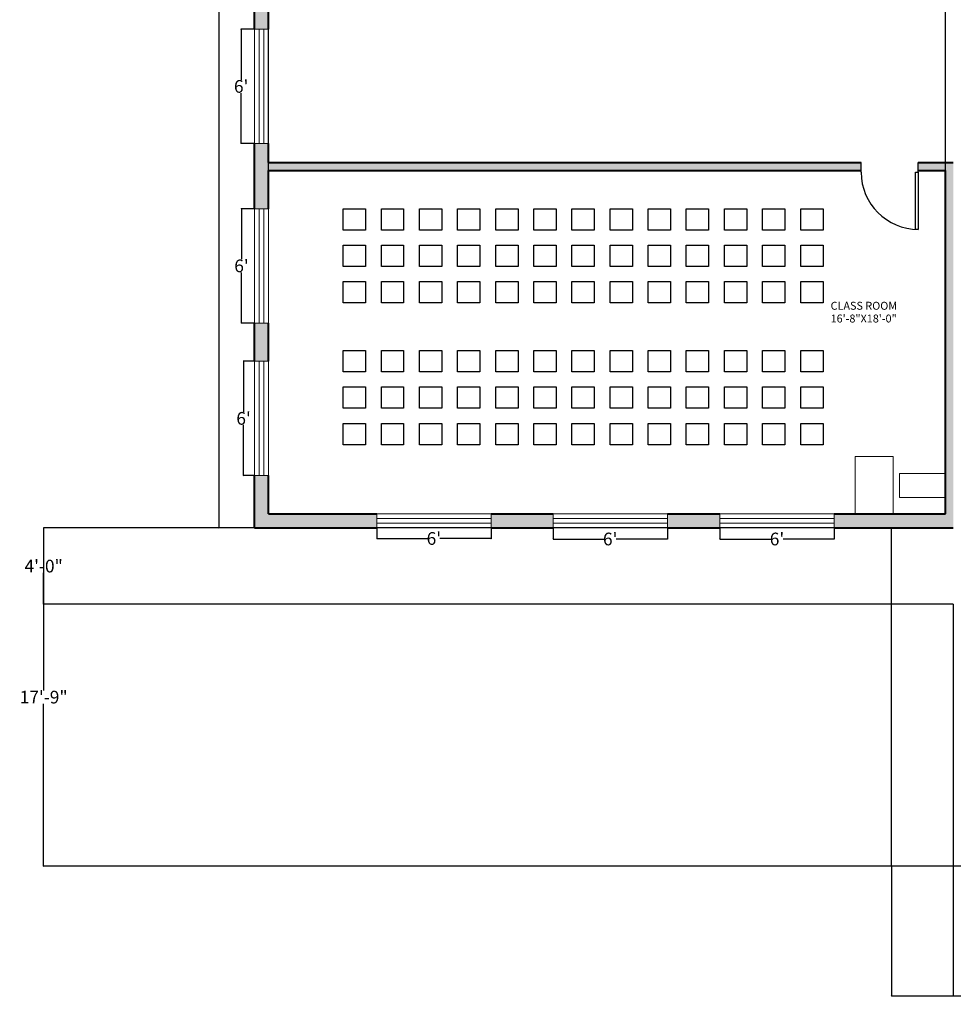
# Model space of a CAD drawing. Units: inches. Extents: x -405 to 940, y 226 to 2032.
# Tile 1 of 10: x -405 to 183, y 226 to 846. Entities that reach past the tile are written whole.
import ezdxf

# ---------------------------------------------------------------- set-up
doc = ezdxf.new("R2010")
doc.units = ezdxf.units.IN
doc.header["$MEASUREMENT"] = 0
doc.linetypes.add('ACAD_ISO02W100', pattern=[15, 12, -3])
for name, color, linetype, lineweight in [('A-ANNO-DIMS', 120, 'Continuous', 18), ('A-AREA-IDEN', 32, 'Continuous', 18), ('A-FLOR-EDGE', 3, 'Continuous', 25), ('A-FURN-SEAT', 5, 'Continuous', 18), ('A-GLAZ-HIDN', 1, 'ACAD_ISO02W100', 18), ('A-WALL-PATT', 8, 'Continuous', 13), ('door', 6, 'Continuous', 25), ('tables', 2, 'Continuous', 18), ('wall', 3, 'Continuous', 40), ('window', 1, 'Continuous', 18)]:
    doc.layers.add(name, color=color, linetype=linetype, lineweight=lineweight)
doc.layers.add('beches', color=5, linetype='Continuous')
doc.styles.get("Standard").update_dxf_attribs({"font": 'arial.ttf'})
doc.dimstyles.get("Standard").update_dxf_attribs({"dimtxt": 8, "dimasz": 0.18, "dimexe": 0.18, "dimexo": 0.0625, "dimgap": 0.09, "dimtad": 0, "dimtih": 1, "dimtoh": 1, "dimdec": 0, "dimzin": 0, "dimdsep": 46, "dimlunit": 3, "dimtxsty": 'Standard', "dimblk": 'OBLIQUE', "dimcen": 0.09, "dimadec": 0, "dimazin": 0, "dimtfac": 1, "dimtdec": 0, "dimtofl": 0, "dimtmove": 0, "dimatfit": 3, "dimfxl": 1, "dimtolj": 1, "dimtzin": 0, "dimarcsym": 0})

# ---------------------------------------------------------------- blocks, each defined once
blk = doc.blocks.new('*U4')
for p, q in [((0, 0), (0, -6)), ((36, 0), (36, -6))]:
    blk.add_line(p, q)
blk.add_lwpolyline([(0, 0), (0, 36), (1.75, 36), (1.75, 0)], close=True)
blk.add_arc((0, 0), 36, 0, 90)
blk = doc.blocks.new('*U17')
at = {"layer": 'beches'}
blk.add_lwpolyline([(6.71, -7.02), (-6.71, -7.02), (-6.71, 7.02), (6.71, 7.02)], close=True, dxfattribs=at)
blk = doc.blocks.new('*U18')
at = {"layer": 'A-FURN-SEAT', "transparency": 16777216}
for p in [(-45.84, 288), (-45.84, 288, 12), (-45.84, 288, 24), (-45.84, 288, 36), (-45.84, 288, 48), (-45.84, 288, 60), (-45.84, 288, 72), (-45.84, 288, 84), (-45.84, 288, 96), (-45.84, 288, 108), (-45.84, 288, 120), (-45.84, 288, 132), (-22.92, 288), (-22.92, 288, 12), (-22.92, 288, 24), (-22.92, 288, 36), (-22.92, 288, 48), (-22.92, 288, 60), (-22.92, 288, 72), (-22.92, 288, 84), (-22.92, 288, 96), (-22.92, 288, 108), (-22.92, 288, 120), (-22.92, 288, 132), (0, 288), (0, 288, 12), (0, 288, 24), (0, 288, 36), (0, 288, 48), (0, 288, 60), (0, 288, 72), (0, 288, 84), (0, 288, 96), (0, 288, 108), (0, 288, 120), (0, 288, 132), (-45.84, 264), (-45.84, 264, 12), (-45.84, 264, 24), (-45.84, 264, 36), (-45.84, 264, 48), (-45.84, 264, 60), (-45.84, 264, 72), (-45.84, 264, 84), (-45.84, 264, 96), (-45.84, 264, 108), (-45.84, 264, 120), (-45.84, 264, 132), (-22.92, 264), (-22.92, 264, 12), (-22.92, 264, 24), (-22.92, 264, 36), (-22.92, 264, 48), (-22.92, 264, 60), (-22.92, 264, 72), (-22.92, 264, 84), (-22.92, 264, 96), (-22.92, 264, 108), (-22.92, 264, 120), (-22.92, 264, 132), (0, 264), (0, 264, 12), (0, 264, 24), (0, 264, 36), (0, 264, 48), (0, 264, 60), (0, 264, 72), (0, 264, 84), (0, 264, 96), (0, 264, 108), (0, 264, 120), (0, 264, 132), (-45.84, 240), (-45.84, 240, 12), (-45.84, 240, 24), (-45.84, 240, 36), (-45.84, 240, 48), (-45.84, 240, 60), (-45.84, 240, 72), (-45.84, 240, 84), (-45.84, 240, 96), (-45.84, 240, 108), (-45.84, 240, 120), (-45.84, 240, 132), (-22.92, 240), (-22.92, 240, 12), (-22.92, 240, 24), (-22.92, 240, 36), (-22.92, 240, 48), (-22.92, 240, 60), (-22.92, 240, 72), (-22.92, 240, 84), (-22.92, 240, 96), (-22.92, 240, 108), (-22.92, 240, 120), (-22.92, 240, 132), (0, 240), (0, 240, 12), (0, 240, 24), (0, 240, 36), (0, 240, 48), (0, 240, 60), (0, 240, 72), (0, 240, 84), (0, 240, 96), (0, 240, 108), (0, 240, 120), (0, 240, 132), (-45.84, 216), (-45.84, 216, 12), (-45.84, 216, 24), (-45.84, 216, 36), (-45.84, 216, 48), (-45.84, 216, 60), (-45.84, 216, 72), (-45.84, 216, 84), (-45.84, 216, 96), (-45.84, 216, 108), (-45.84, 216, 120), (-45.84, 216, 132), (-22.92, 216), (-22.92, 216, 12), (-22.92, 216, 24), (-22.92, 216, 36), (-22.92, 216, 48), (-22.92, 216, 60), (-22.92, 216, 72), (-22.92, 216, 84), (-22.92, 216, 96), (-22.92, 216, 108), (-22.92, 216, 120), (-22.92, 216, 132), (0, 216), (0, 216, 12), (0, 216, 24), (0, 216, 36), (0, 216, 48), (0, 216, 60), (0, 216, 72), (0, 216, 84), (0, 216, 96), (0, 216, 108), (0, 216, 120), (0, 216, 132), (-45.84, 192), (-45.84, 192, 12), (-45.84, 192, 24), (-45.84, 192, 36), (-45.84, 192, 48), (-45.84, 192, 60), (-45.84, 192, 72), (-45.84, 192, 84), (-45.84, 192, 96), (-45.84, 192, 108), (-45.84, 192, 120), (-45.84, 192, 132), (-22.92, 192), (-22.92, 192, 12), (-22.92, 192, 24), (-22.92, 192, 36), (-22.92, 192, 48), (-22.92, 192, 60), (-22.92, 192, 72), (-22.92, 192, 84), (-22.92, 192, 96), (-22.92, 192, 108), (-22.92, 192, 120), (-22.92, 192, 132), (0, 192), (0, 192, 12), (0, 192, 24), (0, 192, 36), (0, 192, 48), (0, 192, 60), (0, 192, 72), (0, 192, 84), (0, 192, 96), (0, 192, 108), (0, 192, 120), (0, 192, 132), (-45.84, 168), (-45.84, 168, 12), (-45.84, 168, 24), (-45.84, 168, 36), (-45.84, 168, 48), (-45.84, 168, 60), (-45.84, 168, 72), (-45.84, 168, 84), (-45.84, 168, 96), (-45.84, 168, 108), (-45.84, 168, 120), (-45.84, 168, 132), (-22.92, 168), (-22.92, 168, 12), (-22.92, 168, 24), (-22.92, 168, 36), (-22.92, 168, 48), (-22.92, 168, 60), (-22.92, 168, 72), (-22.92, 168, 84), (-22.92, 168, 96), (-22.92, 168, 108), (-22.92, 168, 120), (-22.92, 168, 132), (0, 168), (0, 168, 12), (0, 168, 24), (0, 168, 36), (0, 168, 48), (0, 168, 60), (0, 168, 72), (0, 168, 84), (0, 168, 96), (0, 168, 108), (0, 168, 120), (0, 168, 132), (-45.84, 144), (-45.84, 144, 12), (-45.84, 144, 24), (-45.84, 144, 36), (-45.84, 144, 48), (-45.84, 144, 60), (-45.84, 144, 72), (-45.84, 144, 84), (-45.84, 144, 96), (-45.84, 144, 108), (-45.84, 144, 120), (-45.84, 144, 132), (-22.92, 144), (-22.92, 144, 12), (-22.92, 144, 24), (-22.92, 144, 36), (-22.92, 144, 48), (-22.92, 144, 60), (-22.92, 144, 72), (-22.92, 144, 84), (-22.92, 144, 96), (-22.92, 144, 108), (-22.92, 144, 120), (-22.92, 144, 132), (0, 144), (0, 144, 12), (0, 144, 24), (0, 144, 36), (0, 144, 48), (0, 144, 60), (0, 144, 72), (0, 144, 84), (0, 144, 96), (0, 144, 108), (0, 144, 120), (0, 144, 132), (-45.84, 120), (-45.84, 120, 12), (-45.84, 120, 24), (-45.84, 120, 36), (-45.84, 120, 48), (-45.84, 120, 60), (-45.84, 120, 72), (-45.84, 120, 84), (-45.84, 120, 96), (-45.84, 120, 108), (-45.84, 120, 120), (-45.84, 120, 132), (-22.92, 120), (-22.92, 120, 12), (-22.92, 120, 24), (-22.92, 120, 36), (-22.92, 120, 48), (-22.92, 120, 60), (-22.92, 120, 72), (-22.92, 120, 84), (-22.92, 120, 96), (-22.92, 120, 108), (-22.92, 120, 120), (-22.92, 120, 132), (0, 120), (0, 120, 12), (0, 120, 24), (0, 120, 36), (0, 120, 48), (0, 120, 60), (0, 120, 72), (0, 120, 84), (0, 120, 96), (0, 120, 108), (0, 120, 120), (0, 120, 132), (-45.84, 96), (-45.84, 96, 12), (-45.84, 96, 24), (-45.84, 96, 36), (-45.84, 96, 48), (-45.84, 96, 60), (-45.84, 96, 72), (-45.84, 96, 84), (-45.84, 96, 96), (-45.84, 96, 108), (-45.84, 96, 120), (-45.84, 96, 132), (-22.92, 96), (-22.92, 96, 12), (-22.92, 96, 24), (-22.92, 96, 36), (-22.92, 96, 48), (-22.92, 96, 60), (-22.92, 96, 72), (-22.92, 96, 84), (-22.92, 96, 96), (-22.92, 96, 108), (-22.92, 96, 120), (-22.92, 96, 132), (0, 96), (0, 96, 12), (0, 96, 24), (0, 96, 36), (0, 96, 48), (0, 96, 60), (0, 96, 72), (0, 96, 84), (0, 96, 96), (0, 96, 108), (0, 96, 120), (0, 96, 132), (-45.84, 72), (-45.84, 72, 12), (-45.84, 72, 24), (-45.84, 72, 36), (-45.84, 72, 48), (-45.84, 72, 60), (-45.84, 72, 72), (-45.84, 72, 84), (-45.84, 72, 96), (-45.84, 72, 108), (-45.84, 72, 120), (-45.84, 72, 132), (-22.92, 72), (-22.92, 72, 12), (-22.92, 72, 24), (-22.92, 72, 36), (-22.92, 72, 48), (-22.92, 72, 60), (-22.92, 72, 72), (-22.92, 72, 84), (-22.92, 72, 96), (-22.92, 72, 108), (-22.92, 72, 120), (-22.92, 72, 132), (0, 72), (0, 72, 12), (0, 72, 24), (0, 72, 36), (0, 72, 48), (0, 72, 60), (0, 72, 72), (0, 72, 84), (0, 72, 96), (0, 72, 108), (0, 72, 120), (0, 72, 132), (-45.84, 48), (-45.84, 48, 12), (-45.84, 48, 24), (-45.84, 48, 36), (-45.84, 48, 48), (-45.84, 48, 60), (-45.84, 48, 72), (-45.84, 48, 84), (-45.84, 48, 96), (-45.84, 48, 108), (-45.84, 48, 120), (-45.84, 48, 132), (-22.92, 48), (-22.92, 48, 12), (-22.92, 48, 24), (-22.92, 48, 36), (-22.92, 48, 48), (-22.92, 48, 60), (-22.92, 48, 72), (-22.92, 48, 84), (-22.92, 48, 96), (-22.92, 48, 108), (-22.92, 48, 120), (-22.92, 48, 132), (0, 48), (0, 48, 12), (0, 48, 24), (0, 48, 36), (0, 48, 48), (0, 48, 60), (0, 48, 72), (0, 48, 84), (0, 48, 96), (0, 48, 108), (0, 48, 120), (0, 48, 132), (-45.84, 24), (-45.84, 24, 12), (-45.84, 24, 24), (-45.84, 24, 36), (-45.84, 24, 48), (-45.84, 24, 60), (-45.84, 24, 72), (-45.84, 24, 84), (-45.84, 24, 96), (-45.84, 24, 108), (-45.84, 24, 120), (-45.84, 24, 132), (-22.92, 24), (-22.92, 24, 12), (-22.92, 24, 24), (-22.92, 24, 36), (-22.92, 24, 48), (-22.92, 24, 60), (-22.92, 24, 72), (-22.92, 24, 84), (-22.92, 24, 96), (-22.92, 24, 108), (-22.92, 24, 120), (-22.92, 24, 132), (0, 24), (0, 24, 12), (0, 24, 24), (0, 24, 36), (0, 24, 48), (0, 24, 60), (0, 24, 72), (0, 24, 84), (0, 24, 96), (0, 24, 108), (0, 24, 120), (0, 24, 132), (-45.84, 0), (-45.84, 0, 12), (-45.84, 0, 24), (-45.84, 0, 36), (-45.84, 0, 48), (-45.84, 0, 60), (-45.84, 0, 72), (-45.84, 0, 84), (-45.84, 0, 96), (-45.84, 0, 108), (-45.84, 0, 120), (-45.84, 0, 132), (-22.92, 0), (-22.92, 0, 12), (-22.92, 0, 24), (-22.92, 0, 36), (-22.92, 0, 48), (-22.92, 0, 60), (-22.92, 0, 72), (-22.92, 0, 84), (-22.92, 0, 96), (-22.92, 0, 108), (-22.92, 0, 120), (-22.92, 0, 132), (0, 0), (0, 0, 12), (0, 0, 24), (0, 0, 36), (0, 0, 48), (0, 0, 60), (0, 0, 72), (0, 0, 84), (0, 0, 96), (0, 0, 108), (0, 0, 120), (0, 0, 132)]:
    blk.add_blockref('*U17', p, dxfattribs=at)
blk = doc.blocks.new('*U15')
at = {"layer": 'beches'}
blk.add_lwpolyline([(6.71, -7.02), (-6.71, -7.02), (-6.71, 7.02), (6.71, 7.02)], close=True, dxfattribs=at)
blk = doc.blocks.new('*U16')
at = {"layer": 'A-FURN-SEAT', "transparency": 16777216}
for p in [(-45.84, 288), (-45.84, 288, 12), (-45.84, 288, 24), (-45.84, 288, 36), (-45.84, 288, 48), (-45.84, 288, 60), (-45.84, 288, 72), (-45.84, 288, 84), (-45.84, 288, 96), (-45.84, 288, 108), (-45.84, 288, 120), (-45.84, 288, 132), (-22.92, 288), (-22.92, 288, 12), (-22.92, 288, 24), (-22.92, 288, 36), (-22.92, 288, 48), (-22.92, 288, 60), (-22.92, 288, 72), (-22.92, 288, 84), (-22.92, 288, 96), (-22.92, 288, 108), (-22.92, 288, 120), (-22.92, 288, 132), (0, 288), (0, 288, 12), (0, 288, 24), (0, 288, 36), (0, 288, 48), (0, 288, 60), (0, 288, 72), (0, 288, 84), (0, 288, 96), (0, 288, 108), (0, 288, 120), (0, 288, 132), (-45.84, 264), (-45.84, 264, 12), (-45.84, 264, 24), (-45.84, 264, 36), (-45.84, 264, 48), (-45.84, 264, 60), (-45.84, 264, 72), (-45.84, 264, 84), (-45.84, 264, 96), (-45.84, 264, 108), (-45.84, 264, 120), (-45.84, 264, 132), (-22.92, 264), (-22.92, 264, 12), (-22.92, 264, 24), (-22.92, 264, 36), (-22.92, 264, 48), (-22.92, 264, 60), (-22.92, 264, 72), (-22.92, 264, 84), (-22.92, 264, 96), (-22.92, 264, 108), (-22.92, 264, 120), (-22.92, 264, 132), (0, 264), (0, 264, 12), (0, 264, 24), (0, 264, 36), (0, 264, 48), (0, 264, 60), (0, 264, 72), (0, 264, 84), (0, 264, 96), (0, 264, 108), (0, 264, 120), (0, 264, 132), (-45.84, 240), (-45.84, 240, 12), (-45.84, 240, 24), (-45.84, 240, 36), (-45.84, 240, 48), (-45.84, 240, 60), (-45.84, 240, 72), (-45.84, 240, 84), (-45.84, 240, 96), (-45.84, 240, 108), (-45.84, 240, 120), (-45.84, 240, 132), (-22.92, 240), (-22.92, 240, 12), (-22.92, 240, 24), (-22.92, 240, 36), (-22.92, 240, 48), (-22.92, 240, 60), (-22.92, 240, 72), (-22.92, 240, 84), (-22.92, 240, 96), (-22.92, 240, 108), (-22.92, 240, 120), (-22.92, 240, 132), (0, 240), (0, 240, 12), (0, 240, 24), (0, 240, 36), (0, 240, 48), (0, 240, 60), (0, 240, 72), (0, 240, 84), (0, 240, 96), (0, 240, 108), (0, 240, 120), (0, 240, 132), (-45.84, 216), (-45.84, 216, 12), (-45.84, 216, 24), (-45.84, 216, 36), (-45.84, 216, 48), (-45.84, 216, 60), (-45.84, 216, 72), (-45.84, 216, 84), (-45.84, 216, 96), (-45.84, 216, 108), (-45.84, 216, 120), (-45.84, 216, 132), (-22.92, 216), (-22.92, 216, 12), (-22.92, 216, 24), (-22.92, 216, 36), (-22.92, 216, 48), (-22.92, 216, 60), (-22.92, 216, 72), (-22.92, 216, 84), (-22.92, 216, 96), (-22.92, 216, 108), (-22.92, 216, 120), (-22.92, 216, 132), (0, 216), (0, 216, 12), (0, 216, 24), (0, 216, 36), (0, 216, 48), (0, 216, 60), (0, 216, 72), (0, 216, 84), (0, 216, 96), (0, 216, 108), (0, 216, 120), (0, 216, 132), (-45.84, 192), (-45.84, 192, 12), (-45.84, 192, 24), (-45.84, 192, 36), (-45.84, 192, 48), (-45.84, 192, 60), (-45.84, 192, 72), (-45.84, 192, 84), (-45.84, 192, 96), (-45.84, 192, 108), (-45.84, 192, 120), (-45.84, 192, 132), (-22.92, 192), (-22.92, 192, 12), (-22.92, 192, 24), (-22.92, 192, 36), (-22.92, 192, 48), (-22.92, 192, 60), (-22.92, 192, 72), (-22.92, 192, 84), (-22.92, 192, 96), (-22.92, 192, 108), (-22.92, 192, 120), (-22.92, 192, 132), (0, 192), (0, 192, 12), (0, 192, 24), (0, 192, 36), (0, 192, 48), (0, 192, 60), (0, 192, 72), (0, 192, 84), (0, 192, 96), (0, 192, 108), (0, 192, 120), (0, 192, 132), (-45.84, 168), (-45.84, 168, 12), (-45.84, 168, 24), (-45.84, 168, 36), (-45.84, 168, 48), (-45.84, 168, 60), (-45.84, 168, 72), (-45.84, 168, 84), (-45.84, 168, 96), (-45.84, 168, 108), (-45.84, 168, 120), (-45.84, 168, 132), (-22.92, 168), (-22.92, 168, 12), (-22.92, 168, 24), (-22.92, 168, 36), (-22.92, 168, 48), (-22.92, 168, 60), (-22.92, 168, 72), (-22.92, 168, 84), (-22.92, 168, 96), (-22.92, 168, 108), (-22.92, 168, 120), (-22.92, 168, 132), (0, 168), (0, 168, 12), (0, 168, 24), (0, 168, 36), (0, 168, 48), (0, 168, 60), (0, 168, 72), (0, 168, 84), (0, 168, 96), (0, 168, 108), (0, 168, 120), (0, 168, 132), (-45.84, 144), (-45.84, 144, 12), (-45.84, 144, 24), (-45.84, 144, 36), (-45.84, 144, 48), (-45.84, 144, 60), (-45.84, 144, 72), (-45.84, 144, 84), (-45.84, 144, 96), (-45.84, 144, 108), (-45.84, 144, 120), (-45.84, 144, 132), (-22.92, 144), (-22.92, 144, 12), (-22.92, 144, 24), (-22.92, 144, 36), (-22.92, 144, 48), (-22.92, 144, 60), (-22.92, 144, 72), (-22.92, 144, 84), (-22.92, 144, 96), (-22.92, 144, 108), (-22.92, 144, 120), (-22.92, 144, 132), (0, 144), (0, 144, 12), (0, 144, 24), (0, 144, 36), (0, 144, 48), (0, 144, 60), (0, 144, 72), (0, 144, 84), (0, 144, 96), (0, 144, 108), (0, 144, 120), (0, 144, 132), (-45.84, 120), (-45.84, 120, 12), (-45.84, 120, 24), (-45.84, 120, 36), (-45.84, 120, 48), (-45.84, 120, 60), (-45.84, 120, 72), (-45.84, 120, 84), (-45.84, 120, 96), (-45.84, 120, 108), (-45.84, 120, 120), (-45.84, 120, 132), (-22.92, 120), (-22.92, 120, 12), (-22.92, 120, 24), (-22.92, 120, 36), (-22.92, 120, 48), (-22.92, 120, 60), (-22.92, 120, 72), (-22.92, 120, 84), (-22.92, 120, 96), (-22.92, 120, 108), (-22.92, 120, 120), (-22.92, 120, 132), (0, 120), (0, 120, 12), (0, 120, 24), (0, 120, 36), (0, 120, 48), (0, 120, 60), (0, 120, 72), (0, 120, 84), (0, 120, 96), (0, 120, 108), (0, 120, 120), (0, 120, 132), (-45.84, 96), (-45.84, 96, 12), (-45.84, 96, 24), (-45.84, 96, 36), (-45.84, 96, 48), (-45.84, 96, 60), (-45.84, 96, 72), (-45.84, 96, 84), (-45.84, 96, 96), (-45.84, 96, 108), (-45.84, 96, 120), (-45.84, 96, 132), (-22.92, 96), (-22.92, 96, 12), (-22.92, 96, 24), (-22.92, 96, 36), (-22.92, 96, 48), (-22.92, 96, 60), (-22.92, 96, 72), (-22.92, 96, 84), (-22.92, 96, 96), (-22.92, 96, 108), (-22.92, 96, 120), (-22.92, 96, 132), (0, 96), (0, 96, 12), (0, 96, 24), (0, 96, 36), (0, 96, 48), (0, 96, 60), (0, 96, 72), (0, 96, 84), (0, 96, 96), (0, 96, 108), (0, 96, 120), (0, 96, 132), (-45.84, 72), (-45.84, 72, 12), (-45.84, 72, 24), (-45.84, 72, 36), (-45.84, 72, 48), (-45.84, 72, 60), (-45.84, 72, 72), (-45.84, 72, 84), (-45.84, 72, 96), (-45.84, 72, 108), (-45.84, 72, 120), (-45.84, 72, 132), (-22.92, 72), (-22.92, 72, 12), (-22.92, 72, 24), (-22.92, 72, 36), (-22.92, 72, 48), (-22.92, 72, 60), (-22.92, 72, 72), (-22.92, 72, 84), (-22.92, 72, 96), (-22.92, 72, 108), (-22.92, 72, 120), (-22.92, 72, 132), (0, 72), (0, 72, 12), (0, 72, 24), (0, 72, 36), (0, 72, 48), (0, 72, 60), (0, 72, 72), (0, 72, 84), (0, 72, 96), (0, 72, 108), (0, 72, 120), (0, 72, 132), (-45.84, 48), (-45.84, 48, 12), (-45.84, 48, 24), (-45.84, 48, 36), (-45.84, 48, 48), (-45.84, 48, 60), (-45.84, 48, 72), (-45.84, 48, 84), (-45.84, 48, 96), (-45.84, 48, 108), (-45.84, 48, 120), (-45.84, 48, 132), (-22.92, 48), (-22.92, 48, 12), (-22.92, 48, 24), (-22.92, 48, 36), (-22.92, 48, 48), (-22.92, 48, 60), (-22.92, 48, 72), (-22.92, 48, 84), (-22.92, 48, 96), (-22.92, 48, 108), (-22.92, 48, 120), (-22.92, 48, 132), (0, 48), (0, 48, 12), (0, 48, 24), (0, 48, 36), (0, 48, 48), (0, 48, 60), (0, 48, 72), (0, 48, 84), (0, 48, 96), (0, 48, 108), (0, 48, 120), (0, 48, 132), (-45.84, 24), (-45.84, 24, 12), (-45.84, 24, 24), (-45.84, 24, 36), (-45.84, 24, 48), (-45.84, 24, 60), (-45.84, 24, 72), (-45.84, 24, 84), (-45.84, 24, 96), (-45.84, 24, 108), (-45.84, 24, 120), (-45.84, 24, 132), (-22.92, 24), (-22.92, 24, 12), (-22.92, 24, 24), (-22.92, 24, 36), (-22.92, 24, 48), (-22.92, 24, 60), (-22.92, 24, 72), (-22.92, 24, 84), (-22.92, 24, 96), (-22.92, 24, 108), (-22.92, 24, 120), (-22.92, 24, 132), (0, 24), (0, 24, 12), (0, 24, 24), (0, 24, 36), (0, 24, 48), (0, 24, 60), (0, 24, 72), (0, 24, 84), (0, 24, 96), (0, 24, 108), (0, 24, 120), (0, 24, 132), (-45.84, 0), (-45.84, 0, 12), (-45.84, 0, 24), (-45.84, 0, 36), (-45.84, 0, 48), (-45.84, 0, 60), (-45.84, 0, 72), (-45.84, 0, 84), (-45.84, 0, 96), (-45.84, 0, 108), (-45.84, 0, 120), (-45.84, 0, 132), (-22.92, 0), (-22.92, 0, 12), (-22.92, 0, 24), (-22.92, 0, 36), (-22.92, 0, 48), (-22.92, 0, 60), (-22.92, 0, 72), (-22.92, 0, 84), (-22.92, 0, 96), (-22.92, 0, 108), (-22.92, 0, 120), (-22.92, 0, 132), (0, 0), (0, 0, 12), (0, 0, 24), (0, 0, 36), (0, 0, 48), (0, 0, 60), (0, 0, 72), (0, 0, 84), (0, 0, 96), (0, 0, 108), (0, 0, 120), (0, 0, 132)]:
    blk.add_blockref('*U15', p, dxfattribs=at)
blk = doc.blocks.new('_Oblique')
at = {"color": 0, "linetype": 'ByBlock', "lineweight": -2}
blk.add_line((-0.5, -0.5), (0.5, 0.5), dxfattribs=at)
blk = doc.blocks.new('*D44')
at = {"layer": 'A-ANNO-DIMS', "color": 0, "lineweight": -2, "transparency": 16777216}
for p, q in [((-257.29, 1887.81), (-279.61, 1887.81)), ((-279.43, 1887.81), (-279.43, 1210.99)), ((-279.43, 525.81), (-279.43, 1202.63)), ((-257.29, 525.81), (-279.61, 525.81))]:
    blk.add_line(p, q, dxfattribs=at)
at = {"layer": 'Defpoints', "color": 0, "transparency": 16777216}
for p in [(-257.23, 1887.81), (-279.43, 525.81), (-257.23, 525.81)]:
    blk.add_point(p, dxfattribs=at)
at = {"layer": 'A-ANNO-DIMS', "color": 0, "lineweight": -2, "transparency": 16777216, "xscale": 0.18, "yscale": 0.18, "zscale": 0.18}
for p, rotation in [((-279.43, 1887.81), 90), ((-279.43, 525.81), 270)]:
    blk.add_blockref('_Oblique', p, dxfattribs=dict(at, rotation=rotation))
at = {"layer": 'A-ANNO-DIMS', "color": 0, "transparency": 16777216, "insert": (-279.43, 1206.81), "char_height": 8, "attachment_point": 5}
blk.add_mtext('\\A1;113\'-6"', dxfattribs=at)
blk = doc.blocks.new('*D47')
at = {"layer": 'A-ANNO-DIMS', "color": 0, "lineweight": -2, "transparency": 16777216}
for p, q in [((-180.23, 525.75), (-180.23, 519.01)), ((-108.23, 525.75), (-108.23, 519.01)), ((-180.23, 519.19), (-148.02, 519.19)), ((-108.23, 519.19), (-140.44, 519.19))]:
    blk.add_line(p, q, dxfattribs=at)
at = {"layer": 'Defpoints', "color": 0, "transparency": 16777216}
for p in [(-180.23, 525.81), (-108.23, 525.81), (-108.23, 519.19)]:
    blk.add_point(p, dxfattribs=at)
at = {"layer": 'A-ANNO-DIMS', "color": 0, "lineweight": -2, "transparency": 16777216, "xscale": 0.18, "yscale": 0.18, "zscale": 0.18, "rotation": 180}
blk.add_blockref('_Oblique', (-180.23, 519.19), dxfattribs=at)
at = {"layer": 'A-ANNO-DIMS', "color": 0, "lineweight": -2, "transparency": 16777216, "xscale": 0.18, "yscale": 0.18, "zscale": 0.18}
blk.add_blockref('_Oblique', (-108.23, 519.19), dxfattribs=at)
at = {"layer": 'A-ANNO-DIMS', "color": 0, "transparency": 16777216, "insert": (-144.23, 519.19), "char_height": 8, "attachment_point": 5}
blk.add_mtext("\\A1;6'", dxfattribs=at)
blk = doc.blocks.new('*D48')
at = {"layer": 'A-ANNO-DIMS', "color": 0, "lineweight": -2, "transparency": 16777216}
for p, q in [((-69.23, 525.75), (-69.23, 518.68)), ((2.77, 525.75), (2.77, 518.68)), ((-69.23, 518.86), (-37.02, 518.86)), ((2.77, 518.86), (-29.44, 518.86))]:
    blk.add_line(p, q, dxfattribs=at)
at = {"layer": 'Defpoints', "color": 0, "transparency": 16777216}
for p in [(-69.23, 525.81), (2.77, 525.81), (2.77, 518.86)]:
    blk.add_point(p, dxfattribs=at)
at = {"layer": 'A-ANNO-DIMS', "color": 0, "lineweight": -2, "transparency": 16777216, "xscale": 0.18, "yscale": 0.18, "zscale": 0.18, "rotation": 180}
blk.add_blockref('_Oblique', (-69.23, 518.86), dxfattribs=at)
at = {"layer": 'A-ANNO-DIMS', "color": 0, "lineweight": -2, "transparency": 16777216, "xscale": 0.18, "yscale": 0.18, "zscale": 0.18}
blk.add_blockref('_Oblique', (2.77, 518.86), dxfattribs=at)
at = {"layer": 'A-ANNO-DIMS', "color": 0, "transparency": 16777216, "insert": (-33.23, 518.86), "char_height": 8, "attachment_point": 5}
blk.add_mtext("\\A1;6'", dxfattribs=at)
blk = doc.blocks.new('*D49')
at = {"layer": 'A-ANNO-DIMS', "color": 0, "lineweight": -2, "transparency": 16777216}
for p, q in [((35.77, 525.75), (35.77, 518.67)), ((107.77, 525.75), (107.77, 518.67)), ((35.77, 518.85), (67.98, 518.85)), ((107.77, 518.85), (75.56, 518.85))]:
    blk.add_line(p, q, dxfattribs=at)
at = {"layer": 'Defpoints', "color": 0, "transparency": 16777216}
for p in [(35.77, 525.81), (107.77, 525.81), (107.77, 518.85)]:
    blk.add_point(p, dxfattribs=at)
at = {"layer": 'A-ANNO-DIMS', "color": 0, "lineweight": -2, "transparency": 16777216, "xscale": 0.18, "yscale": 0.18, "zscale": 0.18, "rotation": 180}
blk.add_blockref('_Oblique', (35.77, 518.85), dxfattribs=at)
at = {"layer": 'A-ANNO-DIMS', "color": 0, "lineweight": -2, "transparency": 16777216, "xscale": 0.18, "yscale": 0.18, "zscale": 0.18}
blk.add_blockref('_Oblique', (107.77, 518.85), dxfattribs=at)
at = {"layer": 'A-ANNO-DIMS', "color": 0, "transparency": 16777216, "insert": (71.77, 518.85), "char_height": 8, "attachment_point": 5}
blk.add_mtext("\\A1;6'", dxfattribs=at)
blk = doc.blocks.new('*D50')
at = {"layer": 'A-ANNO-DIMS', "color": 0, "lineweight": -2, "transparency": 16777216}
for p, q in [((-257.29, 630.81), (-264.22, 630.81)), ((-264.04, 630.81), (-264.04, 598.98)), ((-264.04, 558.81), (-264.04, 590.64)), ((-257.29, 558.81), (-264.22, 558.81))]:
    blk.add_line(p, q, dxfattribs=at)
at = {"layer": 'Defpoints', "color": 0, "transparency": 16777216}
for p in [(-264.04, 630.81), (-257.23, 630.81), (-257.23, 558.81)]:
    blk.add_point(p, dxfattribs=at)
at = {"layer": 'A-ANNO-DIMS', "color": 0, "lineweight": -2, "transparency": 16777216, "xscale": 0.18, "yscale": 0.18, "zscale": 0.18}
for p, rotation in [((-264.04, 630.81), 90), ((-264.04, 558.81), 270)]:
    blk.add_blockref('_Oblique', p, dxfattribs=dict(at, rotation=rotation))
at = {"layer": 'A-ANNO-DIMS', "color": 0, "transparency": 16777216, "insert": (-264.04, 594.81), "char_height": 8, "attachment_point": 5}
blk.add_mtext("\\A1;6'", dxfattribs=at)
blk = doc.blocks.new('*D51')
at = {"layer": 'A-ANNO-DIMS', "color": 0, "lineweight": -2, "transparency": 16777216}
for p, q in [((-257.29, 726.81), (-265.52, 726.81)), ((-265.34, 726.81), (-265.34, 694.98)), ((-265.34, 654.81), (-265.34, 686.64)), ((-257.29, 654.81), (-265.52, 654.81))]:
    blk.add_line(p, q, dxfattribs=at)
at = {"layer": 'Defpoints', "color": 0, "transparency": 16777216}
for p in [(-265.34, 726.81), (-257.23, 726.81), (-257.23, 654.81)]:
    blk.add_point(p, dxfattribs=at)
at = {"layer": 'A-ANNO-DIMS', "color": 0, "lineweight": -2, "transparency": 16777216, "xscale": 0.18, "yscale": 0.18, "zscale": 0.18}
for p, rotation in [((-265.34, 726.81), 90), ((-265.34, 654.81), 270)]:
    blk.add_blockref('_Oblique', p, dxfattribs=dict(at, rotation=rotation))
at = {"layer": 'A-ANNO-DIMS', "color": 0, "transparency": 16777216, "insert": (-265.34, 690.81), "char_height": 8, "attachment_point": 5}
blk.add_mtext("\\A1;6'", dxfattribs=at)
blk = doc.blocks.new('*D52')
at = {"layer": 'A-ANNO-DIMS', "color": 0, "lineweight": -2, "transparency": 16777216}
for p, q in [((-257.29, 839.81), (-265.73, 839.81)), ((-265.55, 839.81), (-265.55, 807.98)), ((-265.55, 767.81), (-265.55, 799.64)), ((-257.29, 767.81), (-265.73, 767.81))]:
    blk.add_line(p, q, dxfattribs=at)
at = {"layer": 'Defpoints', "color": 0, "transparency": 16777216}
for p in [(-265.55, 839.81), (-257.23, 839.81), (-257.23, 767.81)]:
    blk.add_point(p, dxfattribs=at)
at = {"layer": 'A-ANNO-DIMS', "color": 0, "lineweight": -2, "transparency": 16777216, "xscale": 0.18, "yscale": 0.18, "zscale": 0.18}
for p, rotation in [((-265.55, 839.81), 90), ((-265.55, 767.81), 270)]:
    blk.add_blockref('_Oblique', p, dxfattribs=dict(at, rotation=rotation))
at = {"layer": 'A-ANNO-DIMS', "color": 0, "transparency": 16777216, "insert": (-265.55, 803.81), "char_height": 8, "attachment_point": 5}
blk.add_mtext("\\A1;6'", dxfattribs=at)
blk = doc.blocks.new('DESK-24X36IN')
for p, q in [((0, 36), (24, 36)), ((0, 0), (0, 36)), ((24, 36), (24, 0)), ((24, 0), (0, 0))]:
    blk.add_line(p, q)
blk = doc.blocks.new('CHAIR-DESK')
blk.add_lwpolyline([(0, 15.21), (28.97, 15.21), (28.97, 0), (0, 0)], close=True)
blk = doc.blocks.new('WIN-PANE-72IN')
for p, q in [((0, 3), (72, 3)), ((0, 0), (72, 0))]:
    blk.add_line(p, q)
blk = doc.blocks.new('*D97')
at = {"layer": 'A-ANNO-DIMS', "color": 0, "lineweight": -2, "transparency": 16777216}
for p, q in [((143.77, 312.75), (143.77, 230.98)), ((439.77, 312.75), (439.77, 230.98)), ((143.77, 231.16), (277.87, 231.16)), ((439.77, 231.16), (305.67, 231.16))]:
    blk.add_line(p, q, dxfattribs=at)
at = {"layer": 'Defpoints', "color": 0, "transparency": 16777216}
for p in [(143.77, 312.81), (439.77, 312.81), (439.77, 231.16)]:
    blk.add_point(p, dxfattribs=at)
at = {"layer": 'A-ANNO-DIMS', "color": 0, "lineweight": -2, "transparency": 16777216, "xscale": 0.18, "yscale": 0.18, "zscale": 0.18, "rotation": 180}
blk.add_blockref('_Oblique', (143.77, 231.16), dxfattribs=at)
at = {"layer": 'A-ANNO-DIMS', "color": 0, "lineweight": -2, "transparency": 16777216, "xscale": 0.18, "yscale": 0.18, "zscale": 0.18}
blk.add_blockref('_Oblique', (439.77, 231.16), dxfattribs=at)
at = {"layer": 'A-ANNO-DIMS', "color": 0, "transparency": 16777216, "insert": (291.77, 231.16), "char_height": 8, "attachment_point": 5}
blk.add_mtext('\\A1;24\'-8"', dxfattribs=at)
blk = doc.blocks.new('*D98')
at = {"layer": 'A-ANNO-DIMS', "color": 0, "lineweight": -2, "transparency": 16777216}
for p, q in [((143.71, 525.81), (-390.06, 525.81)), ((-389.88, 525.81), (-389.88, 423.48)), ((-389.88, 312.81), (-389.88, 415.14)), ((143.71, 312.81), (-390.06, 312.81))]:
    blk.add_line(p, q, dxfattribs=at)
at = {"layer": 'Defpoints', "color": 0, "transparency": 16777216}
for p in [(-389.88, 525.81), (143.77, 525.81), (143.77, 312.81)]:
    blk.add_point(p, dxfattribs=at)
at = {"layer": 'A-ANNO-DIMS', "color": 0, "lineweight": -2, "transparency": 16777216, "xscale": 0.18, "yscale": 0.18, "zscale": 0.18}
for p, rotation in [((-389.88, 525.81), 90), ((-389.88, 312.81), 270)]:
    blk.add_blockref('_Oblique', p, dxfattribs=dict(at, rotation=rotation))
at = {"layer": 'A-ANNO-DIMS', "color": 0, "transparency": 16777216, "insert": (-389.88, 419.31), "char_height": 8, "attachment_point": 5}
blk.add_mtext('\\A1;17\'-9"', dxfattribs=at)
blk = doc.blocks.new('*D109')
at = {"layer": 'A-ANNO-DIMS', "color": 0, "lineweight": -2, "transparency": 16777216}
for p, q in [((-248.23, 750.87), (-248.23, 2020.64)), ((-248.23, 2020.46), (-49.06, 2020.46)), ((177.77, 2020.46), (-21.4, 2020.46)), ((177.77, 750.87), (177.77, 2020.64))]:
    blk.add_line(p, q, dxfattribs=at)
at = {"layer": 'Defpoints', "color": 0, "transparency": 16777216}
for p in [(177.77, 2020.46), (-248.23, 750.81), (177.77, 750.81)]:
    blk.add_point(p, dxfattribs=at)
at = {"layer": 'A-ANNO-DIMS', "color": 0, "lineweight": -2, "transparency": 16777216, "xscale": 0.18, "yscale": 0.18, "zscale": 0.18, "rotation": 180}
blk.add_blockref('_Oblique', (-248.23, 2020.46), dxfattribs=at)
at = {"layer": 'A-ANNO-DIMS', "color": 0, "lineweight": -2, "transparency": 16777216, "xscale": 0.18, "yscale": 0.18, "zscale": 0.18}
blk.add_blockref('_Oblique', (177.77, 2020.46), dxfattribs=at)
at = {"layer": 'A-ANNO-DIMS', "color": 0, "transparency": 16777216, "insert": (-35.23, 2020.46), "char_height": 8, "attachment_point": 5}
blk.add_mtext('\\A1;35\'-6"', dxfattribs=at)
blk = doc.blocks.new('*D110')
at = {"layer": 'A-ANNO-DIMS', "color": 0, "lineweight": -2, "transparency": 16777216}
for p, q in [((182.77, 477.75), (182.77, 230.98)), ((379.77, 477.75), (379.77, 230.98)), ((182.77, 231.16), (267.81, 231.16)), ((379.77, 231.16), (294.72, 231.16))]:
    blk.add_line(p, q, dxfattribs=at)
at = {"layer": 'Defpoints', "color": 0, "transparency": 16777216}
for p in [(182.77, 477.81), (379.77, 477.81), (379.77, 231.16)]:
    blk.add_point(p, dxfattribs=at)
at = {"layer": 'A-ANNO-DIMS', "color": 0, "lineweight": -2, "transparency": 16777216, "xscale": 0.18, "yscale": 0.18, "zscale": 0.18, "rotation": 180}
blk.add_blockref('_Oblique', (182.77, 231.16), dxfattribs=at)
at = {"layer": 'A-ANNO-DIMS', "color": 0, "lineweight": -2, "transparency": 16777216, "xscale": 0.18, "yscale": 0.18, "zscale": 0.18}
blk.add_blockref('_Oblique', (379.77, 231.16), dxfattribs=at)
at = {"layer": 'A-ANNO-DIMS', "color": 0, "transparency": 16777216, "insert": (281.27, 231.16), "char_height": 8, "attachment_point": 5}
blk.add_mtext('\\A1;16\'-5"', dxfattribs=at)
blk = doc.blocks.new('*D111')
at = {"layer": 'A-ANNO-DIMS', "color": 0, "lineweight": -2, "transparency": 16777216}
for p, q in [((182.71, 525.81), (-390.06, 525.81)), ((-389.88, 525.81), (-389.88, 505.98)), ((-389.88, 477.81), (-389.88, 497.64)), ((182.71, 477.81), (-390.06, 477.81))]:
    blk.add_line(p, q, dxfattribs=at)
at = {"layer": 'Defpoints', "color": 0, "transparency": 16777216}
for p in [(-389.88, 525.81), (182.77, 525.81), (182.77, 477.81)]:
    blk.add_point(p, dxfattribs=at)
at = {"layer": 'A-ANNO-DIMS', "color": 0, "lineweight": -2, "transparency": 16777216, "xscale": 0.18, "yscale": 0.18, "zscale": 0.18}
for p, rotation in [((-389.88, 525.81), 90), ((-389.88, 477.81), 270)]:
    blk.add_blockref('_Oblique', p, dxfattribs=dict(at, rotation=rotation))
at = {"layer": 'A-ANNO-DIMS', "color": 0, "transparency": 16777216, "insert": (-389.88, 501.81), "char_height": 8, "attachment_point": 5}
blk.add_mtext('\\A1;4\'-0"', dxfattribs=at)

msp = doc.modelspace()

# ---------------------------------------------------------------- hatches: boundary and pattern name
at = {"layer": 'A-WALL-PATT'}
h = msp.add_hatch(dxfattribs=at)
h.set_pattern_fill('AR-HBONE', color=256)
h.set_pattern_definition([(45, (599.8442, 904.9158), (0, 5.656854), [12, -4]), (135, (602.6726, 907.744), (4e-16, 5.656854), [12, -4])])
h.paths.add_polyline_path([(-248.23, 1045.81), (-257.23, 1045.81), (-257.23, 964.81), (-248.23, 964.81)], flags=17)
h.paths.add_polyline_path([(-248.23, 851.81), (-39.23, 851.81), (-39.23, 856.81), (-44.23, 856.81), (-248.23, 856.81), (-248.23, 892.81), (-257.23, 892.81), (-257.23, 839.81), (-248.23, 839.81)])
h.paths.add_polyline_path([(-248.23, 750.81), (124.74, 750.81), (124.74, 751.73), (124.74, 755.81), (-248.23, 755.81), (-248.23, 767.81), (-257.23, 767.81), (-257.23, 726.81), (-248.23, 726.81)])
h.paths.add_polyline_path([(-248.23, 654.81), (-257.23, 654.81), (-257.23, 630.81), (-248.23, 630.81)])
h.paths.add_polyline_path([(-180.23, 534.81), (-248.23, 534.81), (-248.23, 558.81), (-257.23, 558.81), (-257.23, 525.81), (-180.23, 525.81)])
h.paths.add_polyline_path([(-69.23, 534.81), (-108.23, 534.81), (-108.23, 525.81), (-69.23, 525.81)])
h.paths.add_polyline_path([(35.77, 534.81), (2.77, 534.81), (2.77, 525.81), (35.77, 525.81)])
h.paths.add_polyline_path([(182.77, 755.81), (160.74, 755.81), (160.74, 750.81), (177.77, 750.81), (177.77, 534.81), (107.77, 534.81), (107.77, 525.81), (182.77, 525.81)])
h.paths.add_polyline_path([(-39.23, 1609.81), (-44.23, 1609.81), (-44.23, 1604.81), (-44.23, 1460.81), (-135.23, 1460.81), (-135.23, 1465.73), (-140.23, 1465.73), (-140.23, 1460.81), (-248.23, 1460.81), (-248.23, 1471.31), (-257.23, 1471.31), (-257.23, 1419.81), (-248.23, 1419.81), (-248.23, 1455.81), (-44.23, 1455.81), (-44.23, 1194.81), (-39.23, 1194.81)])
h.paths.add_polyline_path([(-248.23, 1520.81), (-257.23, 1520.81), (-257.23, 1495.31), (-248.23, 1495.31), (-248.23, 1505.81), (-140.23, 1505.81), (-140.23, 1495.73), (-135.23, 1495.73), (-135.23, 1516.79), (-140.23, 1516.79), (-140.23, 1510.81), (-248.23, 1510.81)], flags=17)
h.paths.add_polyline_path([(-248.23, 1570.31), (-257.23, 1570.31), (-257.23, 1544.81), (-248.23, 1544.81), (-248.23, 1554.81), (-140.23, 1554.81), (-140.23, 1546.79), (-135.23, 1546.79), (-135.23, 1565.08), (-140.23, 1565.08), (-140.23, 1559.81), (-248.23, 1559.81)], flags=17)
h.paths.add_polyline_path([(-248.23, 1615.81), (-257.23, 1615.81), (-257.23, 1594.31), (-248.23, 1594.31), (-248.23, 1604.81), (-140.23, 1604.81), (-140.23, 1595.08), (-135.23, 1595.08), (-135.23, 1604.81), (-80.23, 1604.81), (-80.23, 1609.81), (-248.23, 1609.81)])
h.paths.add_polyline_path([(-248.23, 1783.81), (-235.46, 1783.81), (-235.46, 1788.81), (-248.23, 1788.81), (-248.23, 1878.81), (-237.73, 1878.81), (-237.73, 1887.81), (-257.23, 1887.81), (-257.23, 1687.81), (-248.23, 1687.81), (-248.23, 1693.81), (-136.23, 1693.81), (-136.23, 1698.81), (-248.23, 1698.81)])
h.paths.add_polyline_path([(-188.23, 1887.81), (-213.73, 1887.81), (-213.73, 1878.81), (-203.23, 1878.81), (-203.23, 1788.81), (-205.46, 1788.81), (-205.46, 1783.81), (-186.39, 1783.81), (-186.39, 1788.81), (-198.23, 1788.81), (-198.23, 1878.81), (-188.23, 1878.81)])
h.paths.add_polyline_path([(-139.23, 1887.81), (-164.23, 1887.81), (-164.23, 1878.81), (-154.23, 1878.81), (-154.23, 1788.81), (-156.39, 1788.81), (-156.39, 1783.81), (-138.25, 1783.81), (-138.25, 1788.81), (-149.23, 1788.81), (-149.23, 1878.81), (-139.23, 1878.81)])
h.paths.add_polyline_path([(-89.23, 1887.81), (-115.23, 1887.81), (-115.23, 1878.81), (-105.23, 1878.81), (-105.23, 1788.81), (-108.25, 1788.81), (-108.25, 1783.81), (-86.45, 1783.81), (-86.45, 1788.81), (-100.23, 1788.81), (-100.23, 1878.81), (-89.23, 1878.81)])
h.paths.add_polyline_path([(-36.23, 1887.81), (-65.23, 1887.81), (-65.23, 1878.81), (-54.23, 1878.81), (-54.23, 1788.81), (-56.45, 1788.81), (-56.45, 1783.81), (-54.23, 1783.81), (-54.23, 1698.81), (-100.23, 1698.81), (-100.23, 1693.81), (-49.23, 1693.81), (-49.23, 1698.81), (-49.23, 1878.81), (-36.23, 1878.81)])
h.paths.add_polyline_path([(89.77, 1887.81), (35.77, 1887.81), (35.77, 1878.81), (48.77, 1878.81), (48.77, 1698.81), (-13.23, 1698.81), (-13.23, 1693.81), (53.77, 1693.81), (53.77, 1698.81), (53.77, 1878.81), (89.77, 1878.81)])
h.paths.add_polyline_path([(255.27, 1887.81), (161.77, 1887.81), (161.77, 1878.81), (197.77, 1878.81), (197.77, 1698.81), (89.77, 1698.81), (89.77, 1693.81), (202.77, 1693.81), (202.77, 1698.81), (202.77, 1878.81), (255.27, 1878.81)])
h.paths.add_polyline_path([(375.27, 1887.81), (327.27, 1887.81), (327.27, 1878.81), (375.27, 1878.81)], flags=17)
h.paths.add_polyline_path([(815.77, 1887.81), (447.27, 1887.81), (447.27, 1878.81), (499.77, 1878.81), (499.77, 1698.81), (238.77, 1698.81), (238.77, 1693.81), (504.77, 1693.81), (504.77, 1878.81), (633.77, 1878.81), (633.77, 1646.81), (597.77, 1646.81), (597.77, 1641.81), (602.77, 1641.81), (638.77, 1641.81), (638.77, 1878.81), (806.77, 1878.81), (806.77, 1838.31), (815.77, 1838.31)])
h.paths.add_polyline_path([(815.77, 1766.31), (806.77, 1766.31), (806.77, 1718.31), (815.77, 1718.31)], flags=17)
h.paths.add_polyline_path([(815.77, 1356.31), (806.77, 1356.31), (806.77, 1303.81), (602.77, 1303.81), (597.77, 1303.81), (597.77, 1037.81), (602.77, 1037.81), (602.77, 1298.81), (806.77, 1298.81), (806.77, 1246.31), (815.77, 1246.31)])
h.paths.add_polyline_path([(815.77, 1174.31), (806.77, 1174.31), (806.77, 1126.31), (815.77, 1126.31)], flags=17)
h.paths.add_polyline_path([(815.77, 1054.31), (806.77, 1054.31), (806.77, 1001.81), (796.08, 1001.81), (796.08, 1001.75), (780.86, 1001.75), (602.77, 1001.81), (597.77, 1001.81), (597.77, 892.81), (602.77, 892.81), (602.77, 996.81), (806.77, 996.81), (806.77, 962.81), (815.77, 962.81)])
h.paths.add_polyline_path([(403.77, 534.81), (379.77, 534.81), (379.77, 525.81), (403.77, 525.81)])
h.paths.add_polyline_path([(-39.23, 1158.81), (-44.23, 1158.81), (-248.23, 1158.81), (-248.23, 1194.81), (-257.23, 1194.81), (-257.23, 1117.81), (-248.23, 1117.81), (-248.23, 1153.81), (-44.23, 1153.81), (-44.23, 892.81), (-39.23, 892.81)])
h.paths.add_polyline_path([(-248.23, 1347.81), (-257.23, 1347.81), (-257.23, 1275.81), (-248.23, 1275.81)], flags=17)
h.paths.add_polyline_path([(815.77, 1476.31), (806.77, 1476.31), (806.77, 1428.31), (815.77, 1428.31)], flags=17)
h.paths.add_polyline_path([(815.77, 1646.31), (806.77, 1646.31), (806.77, 1638.65), (806.77, 1605.81), (597.77, 1605.81), (597.77, 1339.81), (602.77, 1339.81), (602.77, 1600.81), (806.77, 1600.81), (806.77, 1548.31), (815.77, 1548.31)])

# ---------------------------------------------------------------- linework, layer by layer
at = {"layer": 'A-FLOR-EDGE'}
for p, q in [((143.77, 312.81), (143.77, 525.81)), ((439.77, 312.81), (143.77, 312.81))]:
    msp.add_line(p, q, dxfattribs=at)
at = {"layer": 'A-GLAZ-HIDN'}
for p, q in [((-248.23, 839.81), (-257.23, 839.81)), ((-248.23, 767.81), (-257.23, 767.81)), ((-248.23, 726.81), (-257.23, 726.81)), ((-248.23, 654.81), (-257.23, 654.81)), ((-248.23, 630.81), (-257.23, 630.81)), ((-248.23, 558.81), (-257.23, 558.81)), ((-180.23, 534.81), (-180.23, 525.81)), ((-108.23, 534.81), (-108.23, 525.81)), ((-69.23, 534.81), (-69.23, 525.81)), ((2.77, 534.81), (2.77, 525.81)), ((35.77, 534.81), (35.77, 525.81)), ((107.77, 534.81), (107.77, 525.81))]:
    msp.add_line(p, q, dxfattribs=at)
at = {"layer": 'door'}
for p, q in [((124.74, 750.81), (124.74, 755.81)), ((124.74, 749.81), (124.74, 751.73)), ((160.74, 750.81), (160.74, 755.81))]:
    msp.add_line(p, q, dxfattribs=at)
at = {"layer": 'wall'}
for p, q in [((-257.23, 839.81), (-257.23, 892.81)), ((-248.23, 839.81), (-248.23, 851.81)), ((-257.23, 726.81), (-257.23, 767.81)), ((-248.23, 755.81), (-248.23, 767.81)), ((-248.23, 755.81), (124.74, 755.81)), ((-248.23, 750.81), (124.74, 750.81)), ((-248.23, 726.81), (-248.23, 750.81)), ((160.74, 755.81), (182.77, 755.81)), ((160.74, 750.81), (177.77, 750.81)), ((177.77, 534.81), (177.77, 750.81)), ((-257.23, 630.81), (-257.23, 654.81)), ((-248.23, 630.81), (-248.23, 654.81)), ((-257.23, 525.81), (-257.23, 558.81)), ((-248.23, 534.81), (-248.23, 558.81)), ((-248.23, 534.81), (-180.23, 534.81)), ((-108.23, 534.81), (-69.23, 534.81)), ((2.77, 534.81), (35.77, 534.81)), ((107.77, 534.81), (177.77, 534.81)), ((-257.23, 525.81), (-180.23, 525.81)), ((-108.23, 525.81), (-69.23, 525.81)), ((2.77, 525.81), (35.77, 525.81)), ((107.77, 525.81), (182.77, 525.81))]:
    msp.add_line(p, q, dxfattribs=at)
at = {"layer": 'window'}
for p, q in [((-257.23, 767.81), (-257.23, 839.81)), ((-248.23, 767.81), (-248.23, 839.81)), ((-257.23, 654.81), (-257.23, 726.81)), ((-248.23, 654.81), (-248.23, 726.81)), ((-257.23, 558.81), (-257.23, 630.81)), ((-248.23, 558.81), (-248.23, 630.81)), ((-108.23, 534.81), (-180.23, 534.81)), ((2.77, 534.81), (-69.23, 534.81)), ((107.77, 534.81), (35.77, 534.81)), ((-108.23, 525.81), (-180.23, 525.81)), ((2.77, 525.81), (-69.23, 525.81)), ((107.77, 525.81), (35.77, 525.81))]:
    msp.add_line(p, q, dxfattribs=at)

# ---------------------------------------------------------------- block references
at = {"layer": 'A-FURN-SEAT'}
for name, p, rotation in [('*U18', (93.72, 720.06), 90), ('*U16', (93.72, 630.79), 90), ('CHAIR-DESK', (177.77, 560.12), 180)]:
    msp.add_blockref(name, p, dxfattribs=dict(at, rotation=rotation))
at = {"layer": 'door', "rotation": 180}
msp.add_blockref('*U4', (160.74, 749.81), dxfattribs=at)
at = {"layer": 'tables', "rotation": 180}
msp.add_blockref('DESK-24X36IN', (144.92, 570.81), dxfattribs=at)
at = {"layer": 'window'}
for p, rotation in [((-251.23, 767.81), 90.00000000000003), ((-251.23, 654.81), 90), ((-254.23, 630.81), 270)]:
    msp.add_blockref('WIN-PANE-72IN', p, dxfattribs=dict(at, rotation=rotation))
for p in [(-180.23, 528.81), (-69.23, 528.81), (35.77, 528.81)]:
    msp.add_blockref('WIN-PANE-72IN', p, dxfattribs=at)

# ---------------------------------------------------------------- texts
at = {"layer": 'A-AREA-IDEN'}
for s, p in [('CLASS ROOM ', (105.53, 663.2)), ('16\'-8"X18\'-0"', (105.53, 655.17))]:
    msp.add_text(s, height=5, dxfattribs=at).set_placement(p)

# ---------------------------------------------------------------- dimensions: what is measured, and where the dimension line sits
at = {"layer": 'A-ANNO-DIMS'}
for base, p1, p2, override, picture, middle in [((177.77, 2020.46), (-248.23, 750.81), (177.77, 750.81), {"dimdec": 1, "dimlfac": 1, "dimrnd": 0, "dimzin": 1, "dimdsep": 46, "dimlunit": 4, "dimfrac": 2}, '*D109', (-35.23, 2020.46)), ((-108.23, 519.19), (-180.23, 525.81), (-108.23, 525.81), {"dimclrd": 0, "dimclre": 0, "dimclrt": 0}, '*D47', (-144.23, 519.19)), ((2.77, 518.86), (-69.23, 525.81), (2.77, 525.81), {"dimclrd": 0, "dimclre": 0, "dimclrt": 0}, '*D48', (-33.23, 518.86)), ((107.77, 518.85), (35.77, 525.81), (107.77, 525.81), {"dimclrd": 0, "dimclre": 0, "dimclrt": 0}, '*D49', (71.77, 518.85)), ((379.77, 231.16), (182.77, 477.81), (379.77, 477.81), {"dimdec": 1, "dimlfac": 1, "dimrnd": 0, "dimzin": 1, "dimdsep": 46, "dimlunit": 4, "dimfrac": 2}, '*D110', (281.27, 231.16)), ((439.77, 231.16), (143.77, 312.81), (439.77, 312.81), {"dimdec": 1, "dimlfac": 1, "dimrnd": 0, "dimzin": 1, "dimdsep": 46, "dimlunit": 4, "dimfrac": 2}, '*D97', (291.77, 231.16))]:
    dim = msp.add_linear_dim(base=base, p1=p1, p2=p2, dimstyle='Standard', override=override, dxfattribs=at)
    dim.commit()
    dim.dimension.update_dxf_attribs({"geometry": picture, "text_midpoint": middle})
for base, p1, p2, override, picture, middle in [((-279.43, 525.81), (-257.23, 1887.81), (-257.23, 525.81), {"dimclrd": 0, "dimclre": 0, "dimclrt": 0}, '*D44', (-279.43, 1206.81)), ((-265.55, 839.81), (-257.23, 767.81), (-257.23, 839.81), {"dimclrd": 0, "dimclre": 0, "dimclrt": 0}, '*D52', (-265.55, 803.81)), ((-265.34, 726.81), (-257.23, 654.81), (-257.23, 726.81), {"dimclrd": 0, "dimclre": 0, "dimclrt": 0}, '*D51', (-265.34, 690.81)), ((-264.04, 630.81), (-257.23, 558.81), (-257.23, 630.81), {"dimclrd": 0, "dimclre": 0, "dimclrt": 0}, '*D50', (-264.04, 594.81)), ((-389.88, 525.81), (143.77, 312.81), (143.77, 525.81), {"dimdec": 1, "dimlfac": 1, "dimrnd": 0, "dimzin": 1, "dimdsep": 46, "dimlunit": 4, "dimfrac": 2}, '*D98', (-389.88, 419.31)), ((-389.88, 525.81), (182.77, 477.81), (182.77, 525.81), {"dimdec": 1, "dimlfac": 1, "dimrnd": 0, "dimzin": 1, "dimdsep": 46, "dimlunit": 4, "dimfrac": 2}, '*D111', (-389.88, 501.81))]:
    dim = msp.add_linear_dim(base=base, p1=p1, p2=p2, angle=90, dimstyle='Standard', override=override, dxfattribs=at)
    dim.commit()
    dim.dimension.update_dxf_attribs({"geometry": picture, "text_midpoint": middle})

doc.saveas('drawing.dxf')
